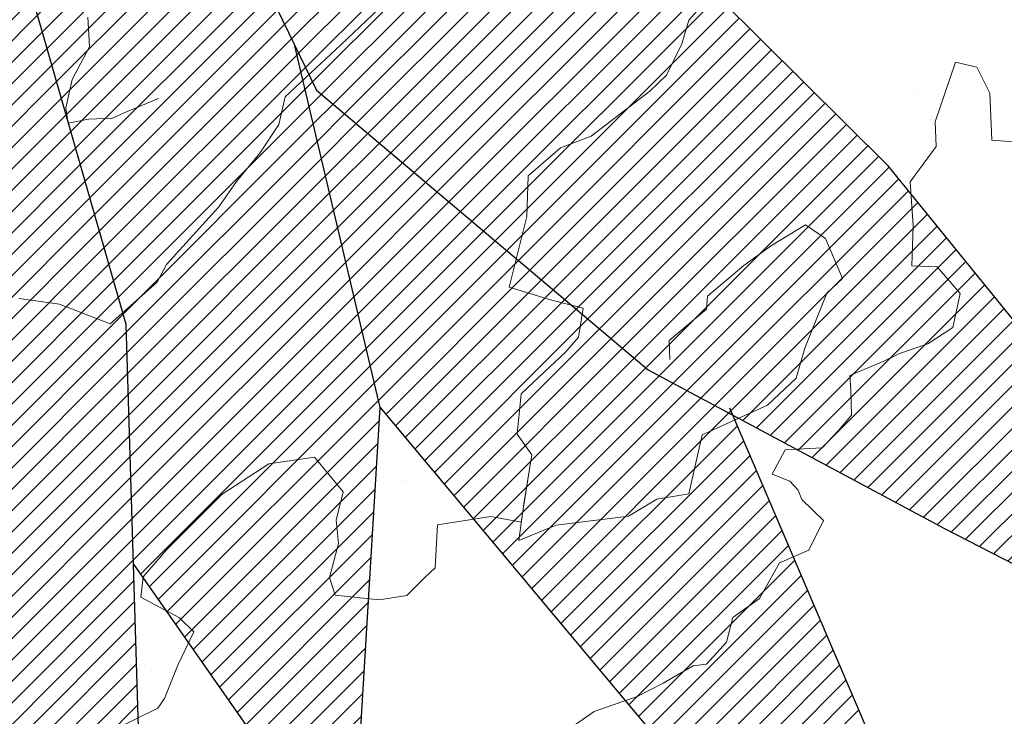
# Model space of a CAD drawing. Units: inches. Extents: x 1986 to 21484, y -1816 to 2016.
# Tile 66 of 85: x 3669.08 to 3679.11, y 1870.8 to 1877.89. Entities that reach past the tile are written whole.
import ezdxf

# ---------------------------------------------------------------- set-up
doc = ezdxf.new("R2010")
doc.units = ezdxf.units.IN
doc.layers.add('L-PLNT', color=84, linetype='Continuous', lineweight=13)
doc.layers.add('vfolhas', color=114, linetype='Continuous', lineweight=5)
for name, color, linetype in [('vfolha', 72, 'Continuous'), ('vfolha2', 110, 'Continuous'), ('vfolhas2', 102, 'Continuous')]:
    doc.layers.add(name, color=color, linetype=linetype)
pattern_1 = [(45, (-2446.5133113, 50.986076), (-0.004419417382, 0.004419417382), [])]

# ---------------------------------------------------------------- blocks, each defined once
blk = doc.blocks.new('arbusto_PB_verde_grande')
at = {"layer": 'vfolha2'}
h = blk.add_hatch(dxfattribs=at)
h.set_pattern_fill('ANSI31', color=256, scale=0.05, style=0)
h.set_pattern_definition(pattern_1)
h.paths.add_polyline_path([(-0.18963, 0.29704), (-0.08553, 0.20192), (-0.10785, 0.25007), (-0.13202, 0.31865), (-0.25096, 0.48479), (-0.44952, 0.5505), (-0.37946, 0.43789)])
h.paths.add_polyline_path([(0.07911, -0.4071), (0.08214, -0.50631), (0.17255, -0.6355), (0.18428, -0.44151), (0.14904, -0.29177), (0.02625, -0.03934), (0.03527, -0.25376)])
at = {"layer": 'vfolhas'}
h = blk.add_hatch(dxfattribs=at)
h.set_pattern_fill('ANSI31', color=256, scale=0.05, style=0)
h.set_pattern_definition(pattern_1)
h.paths.add_polyline_path([(-0.07279, 0.50669), (-0.18085, 0.65063), (-0.2334, 0.67253), (-0.20712, 0.53176), (-0.10785, 0.25007), (0.02625, -0.03934), (0.00028, 0.09048), (0.00816, 0.16241), (-0.04939, 0.29079)])
h.paths.add_polyline_path([(0.09902, 0.41929), (0.09372, 0.26573), (0.07906, 0.18814), (0.15506, 0.36901), (0.26606, 0.5505), (0.28356, 0.63504), (0.2485, 0.68819), (0.25145, 0.63504), (0.20178, 0.54426)])
h.paths.add_polyline_path([(0.12295, 0.24073), (0.047, 0.06233), (0.02625, -0.03934), (0.11122, 0.04358), (0.18428, 0.09364), (0.27478, 0.19376), (0.3215, 0.25323), (0.44129, 0.38467), (0.47634, 0.57866), (0.41789, 0.45347), (0.28939, 0.30954)])
h.paths.add_polyline_path([(0.58145, -0.03779), (0.70707, 0.01536), (0.78591, 0.04667), (0.74796, 0.06549), (0.62818, 0.08423), (0.52595, 0.09048), (0.39745, 0.04358), (0.02625, -0.03934), (0.25728, -0.03154), (0.43834, -0.0347)])
h.paths.add_polyline_path([(0.52022, -0.03647), (0.43834, -0.0347), (0.25728, -0.03154), (0.02625, -0.03934), (0.17964, -0.08515), (0.53768, -0.13167), (0.69541, -0.15357), (0.78591, -0.07852), (0.70413, -0.10042)])
h.paths.add_polyline_path([(0.27189, -0.21929), (0.14922, -0.14107), (0.02625, -0.03934), (0.15794, -0.31007), (0.29522, -0.42585), (0.41789, -0.49157), (0.56396, -0.56669), (0.5114, -0.48532), (0.39456, -0.34139)])
h.paths.add_polyline_path([(-0.05818, -0.47591), (-0.02312, -0.61984), (0.047, -0.80134), (0.08494, -0.59794), (0.07911, -0.4071), (0.03527, -0.25376), (0.02625, -0.03934), (-0.03773, -0.26001)])
h.paths.add_polyline_path([(-0.24218, 0.14054), (-0.11073, 0.06858), (0.02625, -0.03934), (-0.04235, 0.10871), (-0.21007, 0.23757), (-0.36485, 0.33145), (-0.47874, 0.40341), (-0.54303, 0.46288), (-0.49041, 0.33145), (-0.39408, 0.22192)])
h = blk.add_hatch(dxfattribs=at)
h.set_pattern_fill('ANSI31', color=256, scale=0.05, style=0)
h.set_pattern_definition(pattern_1)
h.paths.add_polyline_path([(0.33611, -0.623), (0.43251, -0.67306), (0.39456, -0.59485), (0.3303, -0.44464), (0.29522, -0.42585), (0.15794, -0.31007), (0.14904, -0.29177), (0.18428, -0.44151)])
at = {"layer": 'vfolha'}
for p, q in [((0.39456, -0.34139), (0.27189, -0.21929)), ((0.07911, -0.4071), (0.03527, -0.25376)), ((0.15794, -0.31007), (0.29522, -0.42585)), ((0.5114, -0.48532), (0.39456, -0.34139)), ((0.08494, -0.59794), (0.07911, -0.4071)), ((0.29522, -0.42585), (0.41789, -0.49157)), ((0.41789, -0.49157), (0.56396, -0.56669))]:
    blk.add_line(p, q, dxfattribs=at)
at = {"layer": 'vfolha2'}
for p, q in [((0.02625, -0.03934), (0.15794, -0.31007)), ((0.18428, -0.44151), (0.14904, -0.29177)), ((0.17255, -0.6355), (0.18428, -0.44151)), ((0.08214, -0.50631), (0.17255, -0.6355))]:
    blk.add_line(p, q, dxfattribs=at)
at = {"layer": 'vfolhas2'}
for p, q in [((0.18428, -0.44151), (0.33611, -0.623)), ((0.39456, -0.59485), (0.32904, -0.4417))]:
    blk.add_line(p, q, dxfattribs=at)
blk = doc.blocks.new('PLANT-SHRUB')
for p, q in [((2166.926, 1903.86), (2167.146, 1903.999)), ((2167.146, 1903.999), (2167.447, 1904.021)), ((2167.447, 1904.021), (2167.557, 1903.941)), ((2167.557, 1903.941), (2167.902, 1903.86)), ((2165.577, 1903.772), (2165.892, 1903.889)), ((2165.892, 1903.889), (2166.2, 1903.779)), ((2166.2, 1903.779), (2166.596, 1903.904)), ((2166.596, 1903.904), (2166.926, 1903.86)), ((2166.749, 1903.841), (2166.749, 1903.841)), ((2166.833, 1903.864), (2166.833, 1903.864)), ((2167.041, 1903.837), (2167.041, 1903.837)), ((2167.662, 1903.84), (2167.662, 1903.84)), ((2167.902, 1903.86), (2168.188, 1903.779)), ((2165.577, 1903.772), (2165.577, 1903.772)), ((2165.591, 1903.464), (2165.577, 1903.772)), ((2166.039, 1903.805), (2166.039, 1903.805)), ((2167.366, 1903.794), (2167.366, 1903.794)), ((2167.829, 1903.802), (2167.829, 1903.802)), ((2168.188, 1903.779), (2168.613, 1903.589)), ((2167.908, 1903.723), (2167.908, 1903.723)), ((2168.116, 1903.695), (2168.116, 1903.695)), ((2168.441, 1903.652), (2168.441, 1903.652)), ((2165.642, 1903.599), (2165.642, 1903.599)), ((2166.886, 1903.597), (2166.886, 1903.597)), ((2168.131, 1903.594), (2168.131, 1903.594)), ((2168.613, 1903.589), (2169.031, 1903.53)), ((2165.555, 1903.369), (2165.591, 1903.464)), ((2165.641, 1903.44), (2165.641, 1903.44)), ((2166.242, 1903.44), (2166.242, 1903.44)), ((2167.24, 1903.454), (2167.24, 1903.454)), ((2167.314, 1903.522), (2167.314, 1903.522)), ((2165.555, 1903.244), (2165.555, 1903.369)), ((2167.288, 1903.427), (2167.288, 1903.427)), ((2168.311, 1903.432), (2168.311, 1903.432)), ((2162.98, 1903.039), (2163.272, 1903.237)), ((2163.272, 1903.237), (2163.572, 1903.185)), ((2165.635, 1903.068), (2165.555, 1903.244)), ((2163.572, 1903.185), (2163.851, 1903.061)), ((2164.467, 1902.995), (2164.635, 1903.185)), ((2164.635, 1903.185), (2164.841, 1903.207)), ((2164.841, 1903.207), (2165.083, 1903.222)), ((2165.035, 1903.212), (2165.035, 1903.212)), ((2165.083, 1903.222), (2165.369, 1902.98)), ((2166.28, 1903.21), (2166.28, 1903.21)), ((2167.524, 1903.208), (2167.524, 1903.208)), ((2168.515, 1903.171), (2168.515, 1903.171)), ((2168.769, 1903.206), (2168.769, 1903.206)), ((2162.964, 1902.679), (2162.98, 1903.039)), ((2163.576, 1903.118), (2163.576, 1903.118)), ((2163.62, 1903.041), (2163.62, 1903.041)), ((2163.622, 1903.107), (2163.622, 1903.107)), ((2163.851, 1903.061), (2164.019, 1903.009)), ((2164.655, 1903.079), (2164.655, 1903.079)), ((2164.845, 1903.091), (2164.845, 1903.091)), ((2164.866, 1903.105), (2164.866, 1903.105)), ((2165.22, 1903.054), (2165.22, 1903.054)), ((2165.369, 1902.98), (2165.635, 1903.068)), ((2165.702, 1903.066), (2165.702, 1903.066)), ((2166.111, 1903.103), (2166.111, 1903.103)), ((2166.724, 1903.071), (2166.724, 1903.071)), ((2166.842, 1903.09), (2166.842, 1903.09)), ((2167.356, 1903.1), (2167.356, 1903.1)), ((2168.442, 1903.103), (2168.442, 1903.103)), ((2168.6, 1903.098), (2168.6, 1903.098)), ((2164.019, 1903.009), (2164.371, 1902.878)), ((2164.371, 1902.878), (2164.467, 1902.995)), ((2165.369, 1902.98), (2165.369, 1902.98)), ((2165.369, 1902.98), (2165.369, 1902.98)), ((2165.388, 1903.02), (2165.388, 1903.02)), ((2165.596, 1902.992), (2165.596, 1902.992)), ((2165.921, 1902.949), (2165.921, 1902.949)), ((2167.803, 1903.032), (2167.803, 1903.032)), ((2168.85, 1903.018), (2168.85, 1903.018)), ((2166.464, 1902.878), (2166.464, 1902.878)), ((2166.672, 1902.851), (2166.672, 1902.851)), ((2166.495, 1902.771), (2166.495, 1902.771)), ((2166.997, 1902.808), (2166.997, 1902.808)), ((2167.54, 1902.736), (2167.54, 1902.736)), ((2168.044, 1902.739), (2168.044, 1902.739)), ((2163.147, 1902.496), (2162.964, 1902.679)), ((2163.069, 1902.718), (2163.069, 1902.718)), ((2163.199, 1902.654), (2163.199, 1902.654)), ((2163.273, 1902.722), (2163.273, 1902.722)), ((2164.115, 1902.704), (2164.115, 1902.704)), ((2164.822, 1902.69), (2164.822, 1902.69)), ((2165.137, 1902.709), (2165.137, 1902.709)), ((2166.393, 1902.634), (2165.883, 1902.288)), ((2166.217, 1902.67), (2166.217, 1902.67)), ((2166.393, 1902.634), (2166.393, 1902.634)), ((2166.667, 1902.452), (2166.393, 1902.634)), ((2166.421, 1902.704), (2166.421, 1902.704)), ((2167.263, 1902.657), (2167.263, 1902.657)), ((2167.748, 1902.709), (2167.748, 1902.709)), ((2168.073, 1902.666), (2168.073, 1902.666)), ((2168.285, 1902.662), (2168.285, 1902.662)), ((2164.074, 1902.6), (2164.074, 1902.6)), ((2165.319, 1902.598), (2165.319, 1902.598)), ((2166.564, 1902.596), (2166.564, 1902.596)), ((2167.808, 1902.594), (2167.808, 1902.594)), ((2168.616, 1902.595), (2168.616, 1902.595)), ((2168.824, 1902.567), (2168.824, 1902.567)), ((2169.053, 1902.591), (2169.053, 1902.591)), ((2169.365, 1902.623), (2169.365, 1902.623)), ((2161.373, 1902.455), (2161.676, 1902.121)), ((2162.855, 1902.204), (2163.147, 1902.496)), ((2164.788, 1902.524), (2164.515, 1902.36)), ((2164.788, 1902.524), (2164.788, 1902.524)), ((2165.19, 1902.524), (2164.788, 1902.524)), ((2165.883, 1902.288), (2165.19, 1902.524)), ((2166.667, 1902.452), (2166.667, 1902.452)), ((2166.995, 1902.379), (2166.667, 1902.452)), ((2169.149, 1902.524), (2169.149, 1902.524)), ((2169.692, 1902.453), (2169.692, 1902.453)), ((2163.551, 1902.348), (2163.551, 1902.348)), ((2164.515, 1902.36), (2163.967, 1902.105)), ((2164.474, 1902.371), (2164.474, 1902.371)), ((2166.023, 1902.339), (2166.023, 1902.339)), ((2167.597, 1901.941), (2166.995, 1902.379)), ((2167.622, 1902.353), (2167.622, 1902.353)), ((2167.696, 1902.42), (2167.696, 1902.42)), ((2169.245, 1902.388), (2169.245, 1902.388)), ((2169.9, 1902.426), (2169.9, 1902.426)), ((2163.076, 1902.289), (2163.076, 1902.289)), ((2163.401, 1902.246), (2163.401, 1902.246)), ((2164.4, 1902.304), (2164.4, 1902.304)), ((2164.63, 1902.309), (2164.63, 1902.309)), ((2165.676, 1902.296), (2165.676, 1902.296)), ((2166.699, 1902.3), (2166.699, 1902.3)), ((2167.778, 1902.262), (2167.778, 1902.262)), ((2168.824, 1902.248), (2168.824, 1902.248)), ((2169.847, 1902.253), (2169.847, 1902.253)), ((2162.573, 1901.86), (2162.855, 1902.204)), ((2163.468, 1902.214), (2163.468, 1902.214)), ((2163.944, 1902.175), (2163.944, 1902.175)), ((2164.152, 1902.148), (2164.152, 1902.148)), ((2164.712, 1902.212), (2164.712, 1902.212)), ((2165.957, 1902.209), (2165.957, 1902.209)), ((2167.201, 1902.207), (2167.201, 1902.207)), ((2168.446, 1902.205), (2168.446, 1902.205)), ((2169.691, 1902.203), (2169.691, 1902.203)), ((2161.676, 1902.121), (2161.362, 1901.756)), ((2163.299, 1902.106), (2163.299, 1902.106)), ((2163.75, 1902.105), (2163.597, 1901.691)), ((2163.967, 1902.105), (2163.75, 1902.105)), ((2164.477, 1902.105), (2164.477, 1902.105)), ((2164.544, 1902.104), (2164.544, 1902.104)), ((2165.02, 1902.033), (2165.02, 1902.033)), ((2165.788, 1902.102), (2165.788, 1902.102)), ((2167.033, 1902.1), (2167.033, 1902.1)), ((2168.277, 1902.097), (2168.277, 1902.097)), ((2168.898, 1902.069), (2168.898, 1902.069)), ((2169.522, 1902.095), (2169.522, 1902.095)), ((2163.044, 1901.948), (2163.044, 1901.948)), ((2164.003, 1901.939), (2164.003, 1901.939)), ((2164.09, 1901.934), (2164.09, 1901.934)), ((2165.112, 1901.939), (2165.112, 1901.939)), ((2165.228, 1902.006), (2165.228, 1902.006)), ((2165.553, 1901.963), (2165.553, 1901.963)), ((2165.602, 1901.953), (2165.602, 1901.953)), ((2165.675, 1902.02), (2165.675, 1902.02)), ((2167.225, 1901.988), (2167.225, 1901.988)), ((2167.597, 1901.941), (2167.597, 1901.941)), ((2167.979, 1901.796), (2167.597, 1901.941)), ((2168.824, 1902.002), (2168.824, 1902.002)), ((2162.135, 1901.777), (2162.573, 1901.86)), ((2162.573, 1901.86), (2162.573, 1901.86)), ((2166.096, 1901.892), (2166.096, 1901.892)), ((2166.192, 1901.9), (2166.192, 1901.9)), ((2166.304, 1901.864), (2166.304, 1901.864)), ((2167.238, 1901.887), (2167.238, 1901.887)), ((2168.26, 1901.892), (2168.26, 1901.892)), ((2169.34, 1901.853), (2169.34, 1901.853)), ((2170.386, 1901.84), (2170.386, 1901.84)), ((2161.362, 1901.756), (2161.279, 1901.474)), ((2161.968, 1901.589), (2162.135, 1901.777)), ((2166.629, 1901.821), (2166.629, 1901.821)), ((2167.171, 1901.75), (2167.171, 1901.75)), ((2167.688, 1901.559), (2167.979, 1901.796)), ((2163.597, 1901.691), (2163.651, 1901.448)), ((2163.597, 1901.691), (2163.597, 1901.691)), ((2166.877, 1901.67), (2166.877, 1901.67)), ((2167.379, 1901.723), (2167.379, 1901.723)), ((2167.487, 1901.404), (2167.834, 1901.677)), ((2167.704, 1901.68), (2167.704, 1901.68)), ((2167.834, 1901.677), (2168.02, 1901.424)), ((2168.426, 1901.637), (2168.426, 1901.637)), ((2170.025, 1901.651), (2170.025, 1901.651)), ((2170.099, 1901.719), (2170.099, 1901.719)), ((2161.404, 1901.287), (2161.968, 1901.589)), ((2161.982, 1901.539), (2161.982, 1901.539)), ((2162.503, 1901.573), (2162.503, 1901.573)), ((2162.507, 1901.602), (2162.507, 1901.602)), ((2163.526, 1901.578), (2163.526, 1901.578)), ((2163.581, 1901.553), (2163.581, 1901.553)), ((2163.655, 1901.621), (2163.655, 1901.621)), ((2163.751, 1901.6), (2163.751, 1901.6)), ((2164.605, 1901.539), (2164.605, 1901.539)), ((2164.996, 1901.597), (2164.996, 1901.597)), ((2165.204, 1901.588), (2165.204, 1901.588)), ((2166.241, 1901.595), (2166.241, 1901.595)), ((2166.674, 1901.53), (2166.674, 1901.53)), ((2166.803, 1901.602), (2166.803, 1901.602)), ((2167.287, 1901.249), (2167.688, 1901.559)), ((2167.485, 1901.593), (2167.485, 1901.593)), ((2167.688, 1901.559), (2167.688, 1901.559)), ((2168.247, 1901.608), (2168.247, 1901.608)), ((2168.455, 1901.581), (2168.455, 1901.581)), ((2168.73, 1901.591), (2168.73, 1901.591)), ((2168.78, 1901.538), (2168.78, 1901.538)), ((2169.975, 1901.588), (2169.975, 1901.588)), ((2161.279, 1901.474), (2161.404, 1901.287)), ((2163.651, 1901.448), (2164.048, 1901.367)), ((2163.651, 1901.448), (2163.651, 1901.448)), ((2165.471, 1901.358), (2165.597, 1901.502)), ((2165.597, 1901.502), (2165.597, 1901.502)), ((2165.651, 1901.525), (2165.651, 1901.525)), ((2167.753, 1901.492), (2167.753, 1901.492)), ((2168.799, 1901.478), (2168.799, 1901.478)), ((2169.323, 1901.467), (2169.323, 1901.467)), ((2169.531, 1901.439), (2169.531, 1901.439)), ((2169.822, 1901.483), (2169.822, 1901.483)), ((2170.901, 1901.444), (2170.901, 1901.444)), ((2161.957, 1901.402), (2161.957, 1901.402)), ((2162.5, 1901.33), (2162.5, 1901.33)), ((2164.048, 1901.367), (2164.39, 1901.322)), ((2164.876, 1901.295), (2164.975, 1901.385)), ((2164.975, 1901.385), (2165.471, 1901.358)), ((2165.471, 1901.358), (2165.471, 1901.358)), ((2168.02, 1901.424), (2168.475, 1901.114)), ((2168.475, 1901.114), (2168.79, 1901.415)), ((2168.79, 1901.415), (2168.934, 1901.415)), ((2168.934, 1901.415), (2169.195, 1901.424)), ((2169.195, 1901.424), (2169.429, 1901.262)), ((2169.856, 1901.397), (2169.856, 1901.397)), ((2162.708, 1901.303), (2162.708, 1901.303)), ((2163.033, 1901.26), (2163.033, 1901.26)), ((2164.39, 1901.322), (2164.876, 1901.295)), ((2164.856, 1901.27), (2164.856, 1901.27)), ((2166.405, 1901.238), (2166.405, 1901.238)), ((2167.25, 1900.994), (2167.287, 1901.249)), ((2168.005, 1901.251), (2168.005, 1901.251)), ((2168.078, 1901.319), (2168.078, 1901.319)), ((2169.429, 1901.262), (2169.725, 1900.92)), ((2169.628, 1901.287), (2169.628, 1901.287)), ((2170.399, 1901.325), (2170.399, 1901.325)), ((2170.607, 1901.298), (2170.607, 1901.298)), ((2170.932, 1901.255), (2170.932, 1901.255)), ((2160.917, 1901.211), (2160.917, 1901.211)), ((2161.561, 1901.153), (2161.561, 1901.153)), ((2161.634, 1901.221), (2161.634, 1901.221)), ((2161.9, 1901.215), (2161.9, 1901.215)), ((2161.939, 1901.216), (2161.939, 1901.216)), ((2163.018, 1901.177), (2163.018, 1901.177)), ((2163.145, 1901.213), (2163.145, 1901.213)), ((2163.183, 1901.189), (2163.183, 1901.189)), ((2163.575, 1901.189), (2163.575, 1901.189)), ((2163.783, 1901.161), (2163.783, 1901.161)), ((2164.065, 1901.164), (2164.065, 1901.164)), ((2164.389, 1901.211), (2164.389, 1901.211)), ((2164.783, 1901.202), (2164.783, 1901.202)), ((2165.087, 1901.169), (2165.087, 1901.169)), ((2165.634, 1901.208), (2165.634, 1901.208)), ((2166.166, 1901.13), (2166.166, 1901.13)), ((2166.879, 1901.206), (2166.879, 1901.206)), ((2168.123, 1901.204), (2168.123, 1901.204)), ((2169.368, 1901.202), (2169.368, 1901.202)), ((2170.613, 1901.199), (2170.613, 1901.199)), ((2161.732, 1901.108), (2161.732, 1901.108)), ((2162.976, 1901.106), (2162.976, 1901.106)), ((2164.108, 1901.118), (2164.108, 1901.118)), ((2164.221, 1901.103), (2164.221, 1901.103)), ((2164.651, 1901.047), (2164.651, 1901.047)), ((2165.465, 1901.101), (2165.465, 1901.101)), ((2166.71, 1901.099), (2166.71, 1901.099)), ((2167.213, 1901.117), (2167.213, 1901.117)), ((2167.955, 1901.097), (2167.955, 1901.097)), ((2168.235, 1901.122), (2168.235, 1901.122)), ((2169.199, 1901.094), (2169.199, 1901.094)), ((2169.314, 1901.083), (2169.314, 1901.083)), ((2170.361, 1901.069), (2170.361, 1901.069)), ((2170.444, 1901.092), (2170.444, 1901.092)), ((2164.859, 1901.02), (2164.859, 1901.02)), ((2165.184, 1900.977), (2165.184, 1900.977)), ((2166.94, 1900.721), (2167.25, 1900.994)), ((2167.25, 1900.994), (2167.25, 1900.994)), ((2167.25, 1900.994), (2167.25, 1900.994)), ((2169.28, 1900.968), (2169.28, 1900.968)), ((2170.829, 1900.936), (2170.829, 1900.936)), ((2162.836, 1900.87), (2162.836, 1900.87)), ((2164.385, 1900.838), (2164.385, 1900.838)), ((2165.727, 1900.905), (2165.727, 1900.905)), ((2165.935, 1900.878), (2165.935, 1900.878)), ((2165.984, 1900.851), (2165.984, 1900.851)), ((2166.058, 1900.919), (2166.058, 1900.919)), ((2166.26, 1900.835), (2166.26, 1900.835)), ((2167.607, 1900.887), (2167.607, 1900.887)), ((2169.206, 1900.901), (2169.206, 1900.901)), ((2169.725, 1900.92), (2169.645, 1900.75)), ((2161.432, 1900.816), (2161.432, 1900.816)), ((2162.478, 1900.803), (2162.478, 1900.803)), ((2162.762, 1900.802), (2162.762, 1900.802)), ((2163.5, 1900.808), (2163.5, 1900.808)), ((2164.58, 1900.769), (2164.58, 1900.769)), ((2165.626, 1900.755), (2165.626, 1900.755)), ((2166.648, 1900.76), (2166.648, 1900.76)), ((2166.803, 1900.764), (2166.803, 1900.764)), ((2167.011, 1900.736), (2167.011, 1900.736)), ((2169.645, 1900.75), (2169.339, 1900.561)), ((2165.883, 1900.52), (2166.12, 1900.702)), ((2166.12, 1900.702), (2166.32, 1900.721)), ((2166.32, 1900.721), (2166.612, 1900.721)), ((2166.612, 1900.721), (2166.94, 1900.721)), ((2166.94, 1900.721), (2166.94, 1900.721)), ((2167.336, 1900.694), (2167.336, 1900.694)), ((2167.728, 1900.721), (2167.728, 1900.721)), ((2168.774, 1900.708), (2168.774, 1900.708)), ((2169.796, 1900.713), (2169.796, 1900.713)), ((2170.876, 1900.674), (2170.876, 1900.674)), ((2162.184, 1900.601), (2162.184, 1900.601)), ((2163.429, 1900.599), (2163.429, 1900.599)), ((2164.673, 1900.596), (2164.673, 1900.596)), ((2165.918, 1900.594), (2165.918, 1900.594)), ((2167.163, 1900.592), (2167.163, 1900.592)), ((2167.259, 1900.568), (2167.259, 1900.568)), ((2167.879, 1900.622), (2167.879, 1900.622)), ((2168.087, 1900.595), (2168.087, 1900.595)), ((2168.407, 1900.59), (2168.407, 1900.59)), ((2168.412, 1900.552), (2168.412, 1900.552)), ((2168.808, 1900.536), (2168.808, 1900.536)), ((2169.339, 1900.561), (2169.195, 1900.372)), ((2169.652, 1900.587), (2169.652, 1900.587)), ((2170.408, 1900.55), (2170.408, 1900.55)), ((2170.481, 1900.617), (2170.481, 1900.617)), ((2170.896, 1900.585), (2170.896, 1900.585)), ((2161.914, 1900.446), (2161.914, 1900.446)), ((2162.364, 1900.438), (2162.364, 1900.438)), ((2163.963, 1900.452), (2163.963, 1900.452)), ((2164.037, 1900.519), (2164.037, 1900.519)), ((2165.586, 1900.487), (2165.586, 1900.487)), ((2166.065, 1900.229), (2165.883, 1900.52)), ((2167.186, 1900.501), (2167.186, 1900.501)), ((2168.955, 1900.48), (2168.955, 1900.48)), ((2169.163, 1900.453), (2169.163, 1900.453)), ((2171.38, 1900.345), (2171.713, 1900.498)), ((2171.713, 1900.498), (2171.83, 1900.525)), ((2171.83, 1900.525), (2172.337, 1900.371)), ((2162.131, 1900.344), (2162.131, 1900.344)), ((2162.993, 1900.407), (2162.993, 1900.407)), ((2164.039, 1900.394), (2164.039, 1900.394)), ((2165.062, 1900.399), (2165.062, 1900.399)), ((2166.141, 1900.36), (2166.141, 1900.36)), ((2167.187, 1900.347), (2167.187, 1900.347)), ((2168.21, 1900.352), (2168.21, 1900.352)), ((2169.195, 1900.372), (2168.943, 1900.21)), ((2169.488, 1900.41), (2169.488, 1900.41)), ((2170.03, 1900.339), (2170.03, 1900.339)), ((2171.03, 1900.21), (2171.38, 1900.345)), ((2162.339, 1900.317), (2162.339, 1900.317)), ((2162.664, 1900.274), (2162.664, 1900.274)), ((2166.065, 1900.229), (2166.065, 1900.229)), ((2166.284, 1899.846), (2166.065, 1900.229)), ((2169.289, 1900.313), (2169.289, 1900.313)), ((2170.238, 1900.311), (2170.238, 1900.311)), ((2170.335, 1900.299), (2170.335, 1900.299)), ((2170.563, 1900.269), (2170.563, 1900.269)), ((2171.358, 1900.304), (2171.358, 1900.304)), ((2171.683, 1900.266), (2171.683, 1900.266)), ((2162.822, 1900.212), (2162.822, 1900.212)), ((2163.207, 1900.202), (2163.207, 1900.202)), ((2163.415, 1900.175), (2163.415, 1900.175)), ((2163.74, 1900.132), (2163.74, 1900.132)), ((2164.067, 1900.21), (2164.067, 1900.21)), ((2165.239, 1900.168), (2165.239, 1900.168)), ((2165.311, 1900.208), (2165.311, 1900.208)), ((2166.556, 1900.205), (2166.556, 1900.205)), ((2166.788, 1900.136), (2166.788, 1900.136)), ((2167.8, 1900.203), (2167.8, 1900.203)), ((2168.387, 1900.15), (2168.387, 1900.15)), ((2168.461, 1900.217), (2168.461, 1900.217)), ((2168.943, 1900.21), (2168.916, 1899.752)), ((2169.045, 1900.201), (2169.045, 1900.201)), ((2170.01, 1900.185), (2170.01, 1900.185)), ((2170.29, 1900.199), (2170.29, 1900.199)), ((2171.039, 1900.004), (2171.03, 1900.21)), ((2171.106, 1900.197), (2171.106, 1900.197)), ((2171.314, 1900.17), (2171.314, 1900.17)), ((2171.534, 1900.196), (2171.534, 1900.196)), ((2171.609, 1900.199), (2171.609, 1900.199)), ((2171.639, 1900.127), (2171.639, 1900.127)), ((2162.016, 1900.119), (2162.016, 1900.119)), ((2162.453, 1900.033), (2162.453, 1900.033)), ((2162.653, 1900.105), (2162.653, 1900.105)), ((2163.475, 1900.038), (2163.475, 1900.038)), ((2163.566, 1900.087), (2163.566, 1900.087)), ((2163.898, 1900.103), (2163.898, 1900.103)), ((2164.283, 1900.061), (2164.283, 1900.061)), ((2164.491, 1900.033), (2164.491, 1900.033)), ((2165.143, 1900.1), (2165.143, 1900.1)), ((2165.165, 1900.101), (2165.165, 1900.101)), ((2166.387, 1900.098), (2166.387, 1900.098)), ((2167.632, 1900.096), (2167.632, 1900.096)), ((2168.877, 1900.094), (2168.877, 1900.094)), ((2170.121, 1900.091), (2170.121, 1900.091)), ((2171.366, 1900.089), (2171.366, 1900.089)), ((2172.182, 1900.056), (2172.182, 1900.056)), ((2172.39, 1900.028), (2172.39, 1900.028)), ((2164.555, 1899.999), (2164.555, 1899.999)), ((2164.816, 1899.991), (2164.816, 1899.991)), ((2165.601, 1899.985), (2165.601, 1899.985)), ((2166.623, 1899.99), (2166.623, 1899.99)), ((2167.703, 1899.951), (2167.703, 1899.951)), ((2168.749, 1899.938), (2168.749, 1899.938)), ((2169.771, 1899.943), (2169.771, 1899.943)), ((2171.182, 1899.581), (2171.039, 1900.004)), ((2165.359, 1899.919), (2165.359, 1899.919)), ((2165.567, 1899.892), (2165.567, 1899.892)), ((2165.662, 1899.443), (2166.284, 1899.846)), ((2165.892, 1899.849), (2165.892, 1899.849)), ((2169.662, 1899.867), (2169.662, 1899.867)), ((2170.851, 1899.904), (2170.851, 1899.904)), ((2171.211, 1899.834), (2171.211, 1899.834)), ((2171.897, 1899.891), (2171.897, 1899.891)), ((2163.218, 1899.768), (2163.218, 1899.768)), ((2164.767, 1899.736), (2164.767, 1899.736)), ((2166.366, 1899.75), (2166.366, 1899.75)), ((2166.434, 1899.777), (2166.434, 1899.777)), ((2166.44, 1899.818), (2166.44, 1899.818)), ((2166.642, 1899.75), (2166.642, 1899.75)), ((2167.989, 1899.785), (2167.989, 1899.785)), ((2168.916, 1899.752), (2169.303, 1899.483)), ((2169.588, 1899.799), (2169.588, 1899.799)), ((2162.968, 1899.637), (2162.968, 1899.637)), ((2163.144, 1899.701), (2163.144, 1899.701)), ((2164.014, 1899.624), (2164.014, 1899.624)), ((2165.037, 1899.629), (2165.037, 1899.629)), ((2166.967, 1899.707), (2166.967, 1899.707)), ((2167.51, 1899.636), (2167.51, 1899.636)), ((2163.106, 1899.598), (2163.106, 1899.598)), ((2164.351, 1899.596), (2164.351, 1899.596)), ((2165.595, 1899.593), (2165.595, 1899.593)), ((2166.116, 1899.59), (2166.116, 1899.59)), ((2166.84, 1899.591), (2166.84, 1899.591)), ((2167.162, 1899.577), (2167.162, 1899.577)), ((2167.718, 1899.608), (2167.718, 1899.608)), ((2168.043, 1899.566), (2168.043, 1899.566)), ((2168.084, 1899.589), (2168.084, 1899.589)), ((2168.185, 1899.581), (2168.185, 1899.581)), ((2169.264, 1899.543), (2169.264, 1899.543)), ((2169.329, 1899.587), (2169.329, 1899.587)), ((2170.31, 1899.529), (2170.31, 1899.529)), ((2170.574, 1899.584), (2170.574, 1899.584)), ((2171.021, 1899.447), (2171.182, 1899.581)), ((2171.333, 1899.534), (2171.333, 1899.534)), ((2171.818, 1899.582), (2171.818, 1899.582)), ((2165.37, 1899.152), (2165.662, 1899.443)), ((2167.641, 1899.467), (2167.641, 1899.467)), ((2168.586, 1899.494), (2168.586, 1899.494)), ((2168.794, 1899.467), (2168.794, 1899.467)), ((2169.119, 1899.424), (2169.119, 1899.424)), ((2169.191, 1899.435), (2169.191, 1899.435)), ((2169.303, 1899.483), (2169.86, 1899.384)), ((2170.661, 1899.411), (2171.021, 1899.447)), ((2170.79, 1899.448), (2170.79, 1899.448)), ((2170.864, 1899.516), (2170.864, 1899.516)), ((2172.412, 1899.495), (2172.412, 1899.495)), ((2172.413, 1899.484), (2172.413, 1899.484)), ((2163.309, 1899.243), (2163.638, 1899.37)), ((2163.638, 1899.37), (2163.875, 1899.37)), ((2163.875, 1899.37), (2164.622, 1899.297)), ((2164.346, 1899.35), (2164.346, 1899.35)), ((2164.419, 1899.418), (2164.419, 1899.418)), ((2165.969, 1899.386), (2165.969, 1899.386)), ((2167.568, 1899.399), (2167.568, 1899.399)), ((2169.662, 1899.352), (2169.662, 1899.352)), ((2169.86, 1899.384), (2170.661, 1899.411)), ((2169.87, 1899.325), (2169.87, 1899.325)), ((2163.091, 1899.115), (2163.309, 1899.243)), ((2163.45, 1899.267), (2163.45, 1899.267)), ((2164.529, 1899.229), (2164.529, 1899.229)), ((2164.622, 1899.297), (2164.932, 1899.17)), ((2170.195, 1899.282), (2170.195, 1899.282)), ((2163.046, 1899.189), (2163.046, 1899.189)), ((2163.371, 1899.146), (2163.371, 1899.146)), ((2163.744, 1899.209), (2163.744, 1899.209)), ((2164.932, 1899.17), (2165.37, 1899.152)), ((2164.988, 1899.207), (2164.988, 1899.207)), ((2165.37, 1899.152), (2165.37, 1899.152)), ((2165.576, 1899.215), (2165.576, 1899.215)), ((2166.233, 1899.205), (2166.233, 1899.205)), ((2166.598, 1899.22), (2166.598, 1899.22)), ((2167.478, 1899.202), (2167.478, 1899.202)), ((2167.677, 1899.181), (2167.677, 1899.181)), ((2168.722, 1899.2), (2168.722, 1899.2)), ((2168.724, 1899.168), (2168.724, 1899.168)), ((2169.746, 1899.173), (2169.746, 1899.173)), ((2169.967, 1899.198), (2169.967, 1899.198)), ((2170.738, 1899.211), (2170.738, 1899.211)), ((2170.826, 1899.134), (2170.826, 1899.134)), ((2170.946, 1899.183), (2170.946, 1899.183)), ((2171.212, 1899.196), (2171.212, 1899.196)), ((2171.271, 1899.141), (2171.271, 1899.141)), ((2172.065, 1899.165), (2172.065, 1899.165)), ((2172.456, 1899.193), (2172.456, 1899.193)), ((2162.689, 1899.079), (2163.091, 1899.115)), ((2163.575, 1899.102), (2163.575, 1899.102)), ((2163.914, 1899.074), (2163.914, 1899.074)), ((2164.122, 1899.047), (2164.122, 1899.047)), ((2164.82, 1899.099), (2164.82, 1899.099)), ((2165.621, 1899.067), (2165.621, 1899.067)), ((2166.065, 1899.097), (2166.065, 1899.097)), ((2167.17, 1899.035), (2167.17, 1899.035)), ((2167.309, 1899.095), (2167.309, 1899.095)), ((2168.554, 1899.093), (2168.554, 1899.093)), ((2168.769, 1899.048), (2168.769, 1899.048)), ((2168.843, 1899.116), (2168.843, 1899.116)), ((2169.798, 1899.09), (2169.798, 1899.09)), ((2170.392, 1899.084), (2170.392, 1899.084)), ((2171.043, 1899.088), (2171.043, 1899.088)), ((2171.814, 1899.069), (2171.814, 1899.069)), ((2171.872, 1899.121), (2171.872, 1899.121)), ((2171.991, 1899.098), (2171.991, 1899.098)), ((2172.022, 1899.042), (2172.022, 1899.042)), ((2172.288, 1899.086), (2172.288, 1899.086)), ((2163.948, 1898.986), (2163.948, 1898.986)), ((2164.447, 1899.004), (2164.447, 1899.004)), ((2164.99, 1898.933), (2164.99, 1898.933)), ((2165.547, 1898.999), (2165.547, 1898.999)), ((2163.989, 1898.854), (2163.989, 1898.854)), ((2165.011, 1898.859), (2165.011, 1898.859)), ((2165.198, 1898.905), (2165.198, 1898.905)), ((2165.523, 1898.863), (2165.523, 1898.863)), ((2166.066, 1898.791), (2166.066, 1898.791)), ((2166.091, 1898.82), (2166.091, 1898.82)), ((2166.274, 1898.764), (2166.274, 1898.764)), ((2166.599, 1898.721), (2166.599, 1898.721)), ((2167.137, 1898.806), (2167.137, 1898.806)), ((2168.159, 1898.811), (2168.159, 1898.811)), ((2169.239, 1898.773), (2169.239, 1898.773)), ((2170.044, 1898.765), (2170.044, 1898.765)), ((2170.285, 1898.759), (2170.285, 1898.759)), ((2171.307, 1898.764), (2171.307, 1898.764)), ((2171.594, 1898.733), (2171.594, 1898.733)), ((2163.6, 1898.667), (2163.6, 1898.667)), ((2165.149, 1898.635), (2165.149, 1898.635)), ((2166.749, 1898.649), (2166.749, 1898.649)), ((2166.822, 1898.716), (2166.822, 1898.716)), ((2167.142, 1898.649), (2167.142, 1898.649)), ((2167.35, 1898.622), (2167.35, 1898.622)), ((2168.371, 1898.684), (2168.371, 1898.684)), ((2169.971, 1898.698), (2169.971, 1898.698)), ((2164.028, 1898.595), (2164.028, 1898.595)), ((2165.272, 1898.593), (2165.272, 1898.593)), ((2166.517, 1898.59), (2166.517, 1898.59)), ((2167.675, 1898.579), (2167.675, 1898.579)), ((2167.762, 1898.588), (2167.762, 1898.588)), ((2169.006, 1898.586), (2169.006, 1898.586)), ((2170.251, 1898.584), (2170.251, 1898.584)), ((2171.496, 1898.581), (2171.496, 1898.581)), ((2164.504, 1898.458), (2164.504, 1898.458)), ((2165.55, 1898.445), (2165.55, 1898.445)), ((2166.573, 1898.45), (2166.573, 1898.45)), ((2168.218, 1898.508), (2168.218, 1898.508)), ((2168.426, 1898.48), (2168.426, 1898.48)), ((2168.751, 1898.438), (2168.751, 1898.438)), ((2167.652, 1898.411), (2167.652, 1898.411)), ((2168.024, 1898.365), (2168.024, 1898.365)), ((2168.698, 1898.398), (2168.698, 1898.398)), ((2169.293, 1898.366), (2169.293, 1898.366)), ((2169.501, 1898.339), (2169.501, 1898.339)), ((2169.573, 1898.333), (2169.573, 1898.333)), ((2169.721, 1898.403), (2169.721, 1898.403)), ((2170.8, 1898.364), (2170.8, 1898.364)), ((2171.172, 1898.347), (2171.172, 1898.347)), ((2171.246, 1898.414), (2171.246, 1898.414)), ((2164.728, 1898.249), (2164.728, 1898.249)), ((2164.802, 1898.316), (2164.802, 1898.316)), ((2166.351, 1898.284), (2166.351, 1898.284)), ((2167.95, 1898.298), (2167.95, 1898.298)), ((2169.826, 1898.296), (2169.826, 1898.296)), ((2170.369, 1898.225), (2170.369, 1898.225)), ((2164.666, 1898.206), (2164.666, 1898.206)), ((2165.91, 1898.204), (2165.91, 1898.204)), ((2167.155, 1898.202), (2167.155, 1898.202)), ((2168.4, 1898.199), (2168.4, 1898.199)), ((2169.644, 1898.197), (2169.644, 1898.197)), ((2170.577, 1898.197), (2170.577, 1898.197)), ((2170.889, 1898.195), (2170.889, 1898.195)), ((2170.902, 1898.154), (2170.902, 1898.154)), ((2164.497, 1898.099), (2164.497, 1898.099)), ((2164.986, 1898.089), (2164.986, 1898.089)), ((2165.742, 1898.096), (2165.742, 1898.096)), ((2166.066, 1898.05), (2166.066, 1898.05)), ((2166.986, 1898.094), (2166.986, 1898.094)), ((2167.112, 1898.036), (2167.112, 1898.036)), ((2168.134, 1898.041), (2168.134, 1898.041)), ((2168.231, 1898.092), (2168.231, 1898.092)), ((2169.476, 1898.09), (2169.476, 1898.09)), ((2170.72, 1898.087), (2170.72, 1898.087)), ((2171.445, 1898.083), (2171.445, 1898.083)), ((2164.622, 1897.946), (2164.622, 1897.946)), ((2164.83, 1897.919), (2164.83, 1897.919)), ((2166.003, 1897.965), (2166.003, 1897.965)), ((2167.552, 1897.933), (2167.552, 1897.933)), ((2169.152, 1897.947), (2169.152, 1897.947)), ((2169.214, 1898.002), (2169.214, 1898.002)), ((2169.225, 1898.015), (2169.225, 1898.015)), ((2170.26, 1897.989), (2170.26, 1897.989)), ((2170.774, 1897.982), (2170.774, 1897.982)), ((2171.282, 1897.994), (2171.282, 1897.994)), ((2165.155, 1897.876), (2165.155, 1897.876)), ((2165.929, 1897.898), (2165.929, 1897.898)), ((2165.697, 1897.805), (2165.697, 1897.805)), ((2165.905, 1897.777), (2165.905, 1897.777)), ((2166.23, 1897.735), (2166.23, 1897.735)), ((2165.525, 1897.675), (2165.525, 1897.675)), ((2166.548, 1897.68), (2166.548, 1897.68)), ((2166.773, 1897.663), (2166.773, 1897.663)), ((2166.981, 1897.636), (2166.981, 1897.636)), ((2167.627, 1897.641), (2167.627, 1897.641)), ((2168.673, 1897.628), (2168.673, 1897.628)), ((2169.696, 1897.633), (2169.696, 1897.633)), ((2170.427, 1897.664), (2170.427, 1897.664)), ((2164.95, 1897.592), (2164.95, 1897.592)), ((2165.532, 1897.533), (2165.532, 1897.533)), ((2166.194, 1897.59), (2166.194, 1897.59)), ((2167.131, 1897.547), (2167.131, 1897.547)), ((2167.205, 1897.615), (2167.205, 1897.615)), ((2167.306, 1897.593), (2167.306, 1897.593)), ((2167.439, 1897.587), (2167.439, 1897.587)), ((2167.849, 1897.522), (2167.849, 1897.522)), ((2168.683, 1897.585), (2168.683, 1897.585)), ((2168.754, 1897.583), (2168.754, 1897.583)), ((2169.928, 1897.583), (2169.928, 1897.583)), ((2170.353, 1897.596), (2170.353, 1897.596)), ((2170.775, 1897.594), (2170.775, 1897.594)), ((2168.057, 1897.494), (2168.057, 1897.494)), ((2168.382, 1897.451), (2168.382, 1897.451)), ((2168.865, 1897.356), (2168.671, 1897.291)), ((2169.502, 1897.338), (2168.865, 1897.356)), ((2169.744, 1896.838), (2169.502, 1897.338)), ((2166.041, 1897.28), (2166.041, 1897.28)), ((2167.087, 1897.266), (2167.087, 1897.266)), ((2167.88, 1897.227), (2167.573, 1897.162)), ((2168.671, 1897.291), (2167.88, 1897.227)), ((2168.109, 1897.271), (2168.109, 1897.271)), ((2169.955, 1897.232), (2169.955, 1897.232)), ((2170.001, 1897.238), (2170.001, 1897.238)), ((2170.235, 1897.219), (2170.235, 1897.219)), ((2165.184, 1897.215), (2165.184, 1897.215)), ((2165.587, 1897.203), (2165.587, 1897.203)), ((2166.733, 1897.183), (2166.733, 1897.183)), ((2166.832, 1897.201), (2166.832, 1897.201)), ((2167.573, 1897.162), (2167.202, 1897.114)), ((2170.209, 1897.211), (2170.209, 1897.211)), ((2170.534, 1897.168), (2170.534, 1897.168)), ((2170.566, 1897.194), (2170.566, 1897.194)), ((2165.419, 1897.096), (2165.419, 1897.096)), ((2166.863, 1897.033), (2166.621, 1896.872)), ((2166.664, 1897.093), (2166.664, 1897.093)), ((2167.202, 1897.114), (2166.863, 1897.033)), ((2170.397, 1897.087), (2170.397, 1897.087)), ((2165.846, 1896.872), (2165.313, 1896.872)), ((2165.5, 1896.905), (2165.5, 1896.905)), ((2166.265, 1896.872), (2165.846, 1896.872)), ((2166.621, 1896.872), (2166.265, 1896.872)), ((2166.385, 1896.864), (2166.385, 1896.864)), ((2166.522, 1896.91), (2166.522, 1896.91)), ((2167.602, 1896.871), (2167.602, 1896.871)), ((2170.002, 1896.515), (2169.744, 1896.838)), ((2165.862, 1896.748), (2165.862, 1896.748)), ((2166.312, 1896.797), (2166.312, 1896.797)), ((2166.405, 1896.677), (2166.405, 1896.677)), ((2166.613, 1896.649), (2166.613, 1896.649)), ((2165.871, 1896.589), (2165.871, 1896.589)), ((2166.938, 1896.607), (2166.938, 1896.607)), ((2167.116, 1896.586), (2167.116, 1896.586)), ((2167.481, 1896.535), (2167.481, 1896.535)), ((2166.015, 1896.51), (2166.015, 1896.51)), ((2167.062, 1896.496), (2167.062, 1896.496)), ((2167.513, 1896.446), (2167.513, 1896.446)), ((2167.587, 1896.513), (2167.587, 1896.513)), ((2167.689, 1896.508), (2167.689, 1896.508)), ((2166.497, 1896.14), (2166.497, 1896.14)), ((2166.509, 1896.2), (2166.509, 1896.2)), ((2167.754, 1896.198), (2167.754, 1896.198)), ((2166.341, 1896.093), (2166.341, 1896.093)), ((2167.115, 1896.081), (2167.115, 1896.081)), ((2167.577, 1896.101), (2167.577, 1896.101)), ((2167.585, 1896.09), (2167.585, 1896.09)), ((2167.93, 1895.87), (2167.574, 1896.002)), ((2168.053, 1895.829), (2167.93, 1895.87)), ((2168.236, 1895.667), (2168.053, 1895.829)), ((2166.768, 1895.763), (2166.768, 1895.763)), ((2167.036, 1895.726), (2167.036, 1895.726)), ((2168.059, 1895.731), (2168.059, 1895.731)), ((2168.419, 1895.555), (2168.236, 1895.667)), ((2167.112, 1895.549), (2167.112, 1895.549)), ((2167.32, 1895.522), (2167.32, 1895.522)), ((2168.038, 1895.583), (2168.038, 1895.583)), ((2168.327, 1895.423), (2168.419, 1895.555)), ((2168.419, 1895.555), (2168.419, 1895.555)), ((2167.645, 1895.479), (2167.645, 1895.479)), ((2168.083, 1895.26), (2168.327, 1895.423)), ((2167.727, 1895.138), (2168.083, 1895.26)), ((2167.534, 1894.905), (2167.727, 1895.138))]:
    blk.add_line(p, q)

msp = doc.modelspace()

# ---------------------------------------------------------------- block references
at = {"layer": 'L-PLNT', "rotation": 223.1883365522388}
msp.add_blockref('PLANT-SHRUB', (3953.27, 4742.965), dxfattribs=at)
at = {"layer": 'L-PLNT', "xscale": 24.60366729364114, "yscale": 24.60366729364114, "zscale": 24.60366729364114}
msp.add_blockref('arbusto_PB_verde_grande', (3668.218, 1884.805), dxfattribs=at)

doc.saveas('drawing.dxf')
